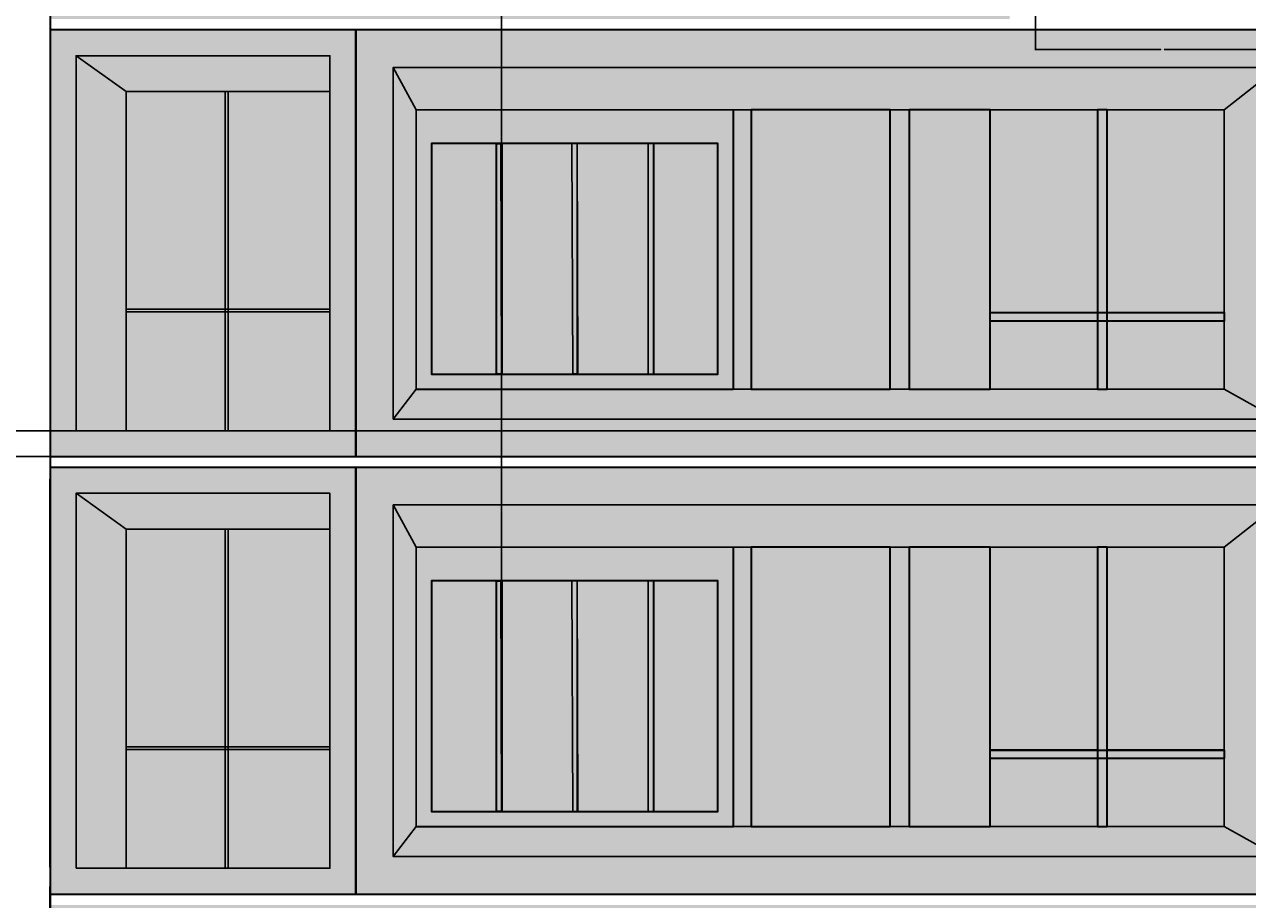
# Model space of a CAD drawing. Units: feet. Extents: x 1141 to 2858, y 751 to 1654.
# Tile 5 of 13: x 1718 to 2096, y 1195 to 1466. Entities that reach past the tile are written whole.
import ezdxf

# ---------------------------------------------------------------- set-up
doc = ezdxf.new("R2010")
doc.units = ezdxf.units.FT
for name, color, linetype, lineweight in [('A-ANNO-DIMS', 2, 'Continuous', 18), ('A-ELEV', 7, 'Continuous', 35), ('A-ELEV-PATT', 8, 'Continuous', 13), ('A-GLAZ', 4, 'Continuous', 25)]:
    doc.layers.add(name, color=color, linetype=linetype, lineweight=lineweight)
doc.styles.get("Standard").update_dxf_attribs({"font": 'arial.ttf'})
doc.dimstyles.get("Standard").update_dxf_attribs({"dimtxt": 0.18, "dimasz": 0.18, "dimexe": 0.18, "dimexo": 0.0625, "dimgap": 0.09, "dimtad": 0, "dimtih": 1, "dimtoh": 1, "dimdec": 1, "dimzin": 0, "dimdsep": 46, "dimlunit": 3, "dimtxsty": 'Standard', "dimcen": 0.09, "dimadec": 0, "dimazin": 0, "dimtfac": 1, "dimtdec": 1, "dimtofl": 0, "dimtmove": 0, "dimatfit": 3, "dimfxl": 1, "dimtolj": 1, "dimtzin": 0, "dimarcsym": 0})

# ---------------------------------------------------------------- blocks, each defined once
blk = doc.blocks.new('WIN-SIDE-A')
blk.add_line((63.09, 104.94), (78.57, 116.03))
blk.add_line((63.09, 104.94), (78.57, 116.03))
for points in [[(78.57, 0), (0, 0), (0, 116.03), (78.57, 116.03)], [(78.57, 0), (0, 0), (0, 116.03), (78.57, 116.03)], [(31.54, 104.94), (32.46, 104.94), (32.46, 0), (31.54, 0)], [(0, 37.61), (63.09, 37.61), (63.09, 36.79), (0, 36.79)]]:
    blk.add_lwpolyline(points, close=True)
for points in [[(63.09, 0), (63.09, 104.94), (0, 104.94)], [(63.09, 0), (63.09, 104.94), (0, 104.94)], [(31.54, 37.61), (31.54, 104.94), (32.46, 104.94), (32.46, 37.61)], [(31.54, 36.79), (0, 36.79), (0, 37.61), (31.54, 37.61)], [(32.46, 36.79), (32.46, 0), (31.54, 0), (31.54, 36.79)], [(32.46, 37.61), (63.09, 37.61), (63.09, 36.79), (32.46, 36.79)]]:
    blk.add_lwpolyline(points)
blk = doc.blocks.new('BALCONY-GLAZ-A')
for p, q in [((0, 108.84), (16.63, 95.74)), ((0, 108.84), (16.63, 95.74)), ((266.62, 95.74), (273.67, 108.84)), ((266.62, 95.74), (273.67, 108.84)), ((16.63, 95.74), (16.63, 9.29)), ((16.63, 95.74), (266.62, 95.74)), ((16.63, 95.74), (16.63, 9.29)), ((16.63, 95.74), (266.62, 95.74)), ((266.62, 95.74), (266.62, 9.19)), ((266.62, 95.74), (266.62, 9.19)), ((16.63, 9.29), (0, 0)), ((16.63, 9.29), (0, 0)), ((16.63, 9.29), (266.62, 9.29)), ((16.63, 9.29), (266.62, 9.29)), ((266.62, 9.29), (273.67, 0)), ((266.62, 9.29), (273.67, 0))]:
    blk.add_line(p, q)
for points in [[(0, 108.84), (273.67, 108.84), (273.67, 0), (0, 0)], [(0, 108.84), (273.67, 108.84), (273.67, 0), (0, 0)], [(266.62, 9.19), (168.47, 9.19), (168.47, 95.74), (266.62, 95.74)], [(266.62, 9.19), (168.47, 9.19), (168.47, 95.74), (266.62, 95.74)]]:
    blk.add_lwpolyline(points, close=True)
blk = doc.blocks.new('WIN-SLIDING')
for points in [[(36.16, 23.71), (36.16, 86.44), (39.2, 86.44), (39.2, 23.71)], [(36.16, 23.71), (0, 23.71), (0, 21.05), (36.16, 21.05)], [(39.2, 21.05), (72.32, 21.05), (72.32, 23.71), (39.2, 23.71)], [(39.2, 21.05), (39.2, 0), (36.16, 0), (36.16, 21.05)]]:
    blk.add_lwpolyline(points)
blk = doc.blocks.new('GLAZ-PANEL-A')
blk.add_lwpolyline([(1.57, 71.37), (0, 71.37), (0, 0), (1.57, 0)], close=True)
for points in [[(1.57, 71.37), (23.57, 71.37)], [(1.57, 0), (1.57, 71.37)], [(23.57, 71.37), (23.57, 0)], [(23.57, 0), (1.57, 0)]]:
    blk.add_lwpolyline(points)
blk = doc.blocks.new('*D15')
at = {"layer": 'A-ANNO-DIMS', "color": 0, "lineweight": -2, "transparency": 16777216}
for p, q in [((2030.85, 1475.38), (2030.85, 1457.85)), ((2109.42, 1475.38), (2109.42, 1457.85)), ((2031.03, 1458.03), (2069.61, 1458.03)), ((2109.24, 1458.03), (2070.66, 1458.03))]:
    blk.add_line(p, q, dxfattribs=at)
at = {"layer": 'A-ANNO-DIMS', "color": 0, "transparency": 16777216}
for points in [[(2031.03, 1458.06), (2031.03, 1458), (2030.85, 1458.03)], [(2109.24, 1458.06), (2109.24, 1458), (2109.42, 1458.03)]]:
    blk.add_solid(points, dxfattribs=at)
at = {"layer": 'Defpoints', "color": 0, "transparency": 16777216}
for p in [(2030.85, 1475.44), (2109.42, 1475.44), (2109.42, 1458.03)]:
    blk.add_point(p, dxfattribs=at)
at = {"layer": 'A-ANNO-DIMS', "color": 0, "transparency": 16777216, "insert": (2070.14, 1458.03), "char_height": 0.18, "attachment_point": 5}
blk.add_mtext('\\A1;79 TYP.', dxfattribs=at)
blk = doc.blocks.new('*D24')
at = {"layer": 'A-ANNO-DIMS', "color": 0, "lineweight": -2, "transparency": 16777216}
for p, q in [((1725.97, 1599.45), (1668.14, 1599.45)), ((1668.32, 1599.27), (1668.32, 1202.86)), ((1668.32, 806.08), (1668.32, 1202.49)), ((1725.97, 805.9), (1668.14, 805.9))]:
    blk.add_line(p, q, dxfattribs=at)
at = {"layer": 'A-ANNO-DIMS', "color": 0, "transparency": 16777216}
for points in [[(1668.29, 1599.27), (1668.35, 1599.27), (1668.32, 1599.45)], [(1668.29, 806.08), (1668.35, 806.08), (1668.32, 805.9)]]:
    blk.add_solid(points, dxfattribs=at)
at = {"layer": 'Defpoints', "color": 0, "transparency": 16777216}
for p in [(1668.32, 1599.45), (1726.03, 1599.45), (1726.03, 805.9)]:
    blk.add_point(p, dxfattribs=at)
at = {"layer": 'A-ANNO-DIMS', "color": 0, "transparency": 16777216, "insert": (1668.32, 1202.68), "char_height": 0.18, "attachment_point": 5}
blk.add_mtext('\\A1;793.6', dxfattribs=at)
blk = doc.blocks.new('*D39')
at = {"layer": 'A-ANNO-DIMS', "color": 0, "lineweight": -2, "transparency": 16777216}
for p, q in [((2319.24, 1599.45), (1668.14, 1599.45)), ((1668.32, 1599.27), (1668.32, 1202.86)), ((1668.32, 806.08), (1668.32, 1202.49)), ((2319.24, 805.9), (1668.14, 805.9))]:
    blk.add_line(p, q, dxfattribs=at)
at = {"layer": 'A-ANNO-DIMS', "color": 0, "transparency": 16777216}
for points in [[(1668.29, 1599.27), (1668.35, 1599.27), (1668.32, 1599.45)], [(1668.29, 806.08), (1668.35, 806.08), (1668.32, 805.9)]]:
    blk.add_solid(points, dxfattribs=at)
at = {"layer": 'Defpoints', "color": 0, "transparency": 16777216}
for p in [(1668.32, 1599.45), (2319.3, 1599.45), (2319.3, 805.9)]:
    blk.add_point(p, dxfattribs=at)
at = {"layer": 'A-ANNO-DIMS', "color": 0, "transparency": 16777216, "insert": (1668.32, 1202.68), "char_height": 0.18, "attachment_point": 5}
blk.add_mtext('\\A1;793.6', dxfattribs=at)
blk = doc.blocks.new('*D54')
at = {"layer": 'A-ANNO-DIMS', "color": 0, "lineweight": -2, "transparency": 16777216}
for p, q in [((2327.22, 1340.05), (1668.14, 1340.05)), ((1668.32, 1339.87), (1668.32, 1336.24)), ((1668.32, 1332.24), (1668.32, 1335.88)), ((2319.24, 1332.06), (1668.14, 1332.06))]:
    blk.add_line(p, q, dxfattribs=at)
at = {"layer": 'A-ANNO-DIMS', "color": 0, "transparency": 16777216}
for points in [[(1668.29, 1339.87), (1668.35, 1339.87), (1668.32, 1340.05)], [(1668.29, 1332.24), (1668.35, 1332.24), (1668.32, 1332.06)]]:
    blk.add_solid(points, dxfattribs=at)
at = {"layer": 'Defpoints', "color": 0, "transparency": 16777216}
for p in [(1668.32, 1340.05), (2327.29, 1340.05), (2319.3, 1332.06)]:
    blk.add_point(p, dxfattribs=at)
at = {"layer": 'A-ANNO-DIMS', "color": 0, "transparency": 16777216, "insert": (1668.32, 1336.06), "char_height": 0.18, "attachment_point": 5}
blk.add_mtext('\\A1;7.986', dxfattribs=at)
blk = doc.blocks.new('*D91')
at = {"layer": 'A-ANNO-DIMS', "color": 0, "lineweight": -2, "transparency": 16777216}
for p, q in [((1726.03, 1196.74), (1726.03, 1654.28)), ((1726.21, 1654.1), (1795.4, 1654.1)), ((1865.51, 1654.1), (1796.32, 1654.1)), ((1865.69, 1222.22), (1865.69, 1654.28))]:
    blk.add_line(p, q, dxfattribs=at)
at = {"layer": 'A-ANNO-DIMS', "color": 0, "transparency": 16777216}
for points in [[(1726.21, 1654.13), (1726.21, 1654.07), (1726.03, 1654.1)], [(1865.51, 1654.13), (1865.51, 1654.07), (1865.69, 1654.1)]]:
    blk.add_solid(points, dxfattribs=at)
at = {"layer": 'Defpoints', "color": 0, "transparency": 16777216}
for p in [(1865.69, 1654.1), (1865.69, 1222.16), (1726.03, 1196.68)]:
    blk.add_point(p, dxfattribs=at)
at = {"layer": 'A-ANNO-DIMS', "color": 0, "transparency": 16777216, "insert": (1795.86, 1654.1), "char_height": 0.18, "attachment_point": 5}
blk.add_mtext('\\A1;139.65', dxfattribs=at)

msp = doc.modelspace()

# ---------------------------------------------------------------- hatches: boundary and pattern name
at = {"layer": 'A-ELEV-PATT'}
h = msp.add_hatch(color=256, dxfattribs=at)
h.dxf.hatch_style = 1
h.paths.add_polyline_path([(2206.032, 1599.4527), (2192.689, 1599.4527), (2192.689, 919.339), (2206.032, 919.339)])
h.paths.add_polyline_path([(2190.2416, 1599.4527), (2175.463, 1599.4527), (2175.463, 919.339), (2190.2416, 919.339)])
h.paths.add_polyline_path([(2173.0156, 1599.4527), (2117.407, 1599.4527), (2117.407, 919.339), (2173.0156, 919.339)])
h.paths.add_polyline_path([(2022.8666, 1057.9008), (1726.032, 1057.9008), (1726.032, 925.9008), (2022.8666, 925.9008)])
h.paths.add_polyline_path([(1737.6123, 937.4811), (1737.6123, 1046.3205), (2011.2863, 1046.3205), (2011.2863, 937.4811)], flags=16)
h.paths.add_polyline_path([(1754.2423, 946.7736), (1754.2423, 1033.2183), (2004.2323, 1033.2183), (2004.2323, 946.7736), (2004.3069, 946.6754), (1906.0824, 946.6754)], flags=0)
h.paths.add_polyline_path([(1900.5421, 946.7736), (1857.5566, 946.7736), (1857.5566, 1033.2183), (1900.5421, 1033.2183)], flags=0)
h.paths.add_polyline_path([(1910.8368, 951.4297), (1910.8368, 1022.7957), (1999.478, 1022.7957), (1999.478, 951.4297)], flags=0)
h.paths.add_polyline_path([(1930.8039, 951.4297), (1930.8039, 1022.7957), (1932.373, 1022.7957), (1932.373, 951.4297)], flags=0)
h.paths.add_polyline_path([(1851.6414, 946.7736), (1826.5664, 946.7736), (1826.5664, 967.8234), (1793.4402, 967.8234), (1793.4402, 946.7736), (1790.4043, 946.7736), (1790.4043, 967.8234), (1754.2423, 967.8234), (1754.2423, 970.4796), (1790.4043, 970.4796), (1790.4043, 1033.2183), (1793.4402, 1033.2183), (1793.4402, 970.4796), (1826.5664, 970.4796), (1826.5664, 1033.2183), (1851.6414, 1033.2183)], flags=0)
h.paths.add_polyline_path([(1954.3728, 951.4297), (1954.3728, 1022.7957), (1955.9419, 1022.7957), (1955.9419, 951.4297)], flags=0)
h.paths.add_polyline_path([(1977.7327, 951.4297), (1977.7327, 1022.7957), (1979.3018, 1022.7957), (1979.3018, 951.4297)], flags=0)
h.paths.add_polyline_path([(2022.8666, 1193.2888), (1726.032, 1193.2888), (1726.032, 1061.2888), (2022.8666, 1061.2888)])
h.paths.add_polyline_path([(1737.6123, 1072.869), (1737.6123, 1181.7085), (2011.2863, 1181.7085), (2011.2863, 1072.869)], flags=16)
h.paths.add_polyline_path([(1754.2423, 1082.1616), (1754.2423, 1168.6063), (2004.2323, 1168.6063), (2004.2323, 1082.1616), (2004.3069, 1082.0634), (1906.0824, 1082.0634)], flags=0)
h.paths.add_polyline_path([(1900.5421, 1082.1616), (1857.5566, 1082.1616), (1857.5566, 1168.6063), (1900.5421, 1168.6063)], flags=0)
h.paths.add_polyline_path([(1910.8368, 1086.8177), (1910.8368, 1158.1837), (1999.478, 1158.1837), (1999.478, 1086.8177)], flags=0)
h.paths.add_polyline_path([(1930.8039, 1086.8177), (1930.8039, 1158.1837), (1932.373, 1158.1837), (1932.373, 1086.8177)], flags=0)
h.paths.add_polyline_path([(1851.6414, 1082.1616), (1826.5664, 1082.1616), (1826.5664, 1103.2114), (1793.4402, 1103.2114), (1793.4402, 1082.1616), (1790.4043, 1082.1616), (1790.4043, 1103.2114), (1754.2423, 1103.2114), (1754.2423, 1105.8676), (1790.4043, 1105.8676), (1790.4043, 1168.6063), (1793.4402, 1168.6063), (1793.4402, 1105.8676), (1826.5664, 1105.8676), (1826.5664, 1168.6063), (1851.6414, 1168.6063)], flags=0)
h.paths.add_polyline_path([(1954.3728, 1086.8177), (1954.3728, 1158.1837), (1955.9419, 1158.1837), (1955.9419, 1086.8177)], flags=0)
h.paths.add_polyline_path([(1977.7327, 1086.8177), (1977.7327, 1158.1837), (1979.3018, 1158.1837), (1979.3018, 1086.8177)], flags=0)
h.paths.add_polyline_path([(2022.8666, 1599.4527), (1726.032, 1599.4527), (1726.032, 1467.4527), (2022.8666, 1467.4527)])
h.paths.add_polyline_path([(2011.2863, 1479.033), (1737.6123, 1479.033), (1737.6123, 1587.8725), (2011.2863, 1587.8725)], flags=16)
h.paths.add_polyline_path([(2004.2323, 1488.3255), (1754.2423, 1488.3255), (1754.2423, 1574.7702), (2004.2323, 1574.7702)], flags=0)
h.paths.add_polyline_path([(1829.1345, 1544.6458), (1914.1177, 1544.6458), (1914.1177, 1539.5463), (1830.9097, 1539.5463), (1831.6817, 1537.3286), (1914.1177, 1537.3286), (1914.1177, 1532.2291), (1833.4569, 1532.2291), (1834.229, 1530.0113), (1914.1177, 1530.0113), (1914.1177, 1524.9118), (1836.0042, 1524.9118), (1836.7762, 1522.694), (1914.1177, 1522.694), (1914.1177, 1517.5946), (1838.5514, 1517.5946), (1839.3235, 1515.3768), (1914.1177, 1515.3768), (1914.1177, 1510.2773), (1841.0987, 1510.2773), (1841.8707, 1508.0595), (1914.1177, 1508.0595), (1914.1177, 1502.9601), (1843.6459, 1502.9601), (1844.4179, 1500.7423), (1914.1177, 1500.7423), (1914.1177, 1495.6428), (1846.1931, 1495.6428), (1846.9652, 1493.425), (1914.1177, 1493.425), (1914.1177, 1488.3255), (1848.6593, 1488.3255), (1848.6593, 1488.5583)], flags=0)
h.paths.add_polyline_path([(2117.407, 1464.0647), (1820.5724, 1464.0647), (1820.5724, 1332.0647), (2117.407, 1332.0647)])
h.paths.add_polyline_path([(2105.8267, 1452.4845), (2105.8267, 1343.645), (1832.1527, 1343.645), (1832.1527, 1452.4845)], flags=16)
h.paths.add_polyline_path([(2089.1967, 1439.3822), (2089.1967, 1352.9376), (1937.3566, 1352.9376), (1937.3566, 1352.8393), (1839.1321, 1352.8393), (1839.2067, 1352.9376), (1839.2067, 1439.3822), (1937.3566, 1439.3822)], flags=0)
h.paths.add_polyline_path([(2016.8727, 1439.3822), (2016.8727, 1376.6436), (2049.9988, 1376.6436), (2049.9988, 1439.3822), (2053.0347, 1439.3822), (2053.0347, 1376.6436), (2089.1967, 1376.6436), (2089.1967, 1373.9873), (2053.0347, 1373.9873), (2053.0347, 1352.9376), (2049.9988, 1352.9376), (2049.9988, 1373.9873), (2016.8727, 1373.9873), (2016.8727, 1352.9376), (1991.7976, 1352.9376), (1991.7976, 1439.3822)], flags=0)
h.paths.add_polyline_path([(1985.8824, 1439.3822), (1985.8824, 1352.9376), (1942.8969, 1352.9376), (1942.8969, 1439.3822)], flags=0)
h.paths.add_polyline_path([(1932.6022, 1428.9596), (1932.6022, 1357.5937), (1843.961, 1357.5937), (1843.961, 1428.9596)], flags=0)
h.paths.add_polyline_path([(1912.6351, 1428.9596), (1912.6351, 1357.5937), (1911.066, 1357.5937), (1911.066, 1428.9596)], flags=0)
h.paths.add_polyline_path([(1889.0662, 1428.9596), (1889.0662, 1357.5937), (1887.4971, 1357.5937), (1887.4971, 1428.9596)], flags=0)
h.paths.add_polyline_path([(1865.7063, 1428.9596), (1865.7063, 1357.5937), (1864.1372, 1357.5937), (1864.1372, 1428.9596)], flags=0)
h.paths.add_polyline_path([(2117.407, 1328.6768), (1820.5724, 1328.6768), (1820.5724, 1196.6768), (2117.407, 1196.6768)])
h.paths.add_polyline_path([(2105.8267, 1317.0965), (2105.8267, 1208.257), (1832.1527, 1208.257), (1832.1527, 1317.0965)], flags=16)
h.paths.add_polyline_path([(2089.1967, 1303.9943), (2089.1967, 1217.5496), (1937.3566, 1217.5496), (1937.3566, 1217.4513), (1839.1321, 1217.4513), (1839.2067, 1217.5496), (1839.2067, 1303.9943), (1937.3566, 1303.9943)], flags=0)
h.paths.add_polyline_path([(2016.8727, 1303.9943), (2016.8727, 1241.2556), (2049.9988, 1241.2556), (2049.9988, 1303.9943), (2053.0347, 1303.9943), (2053.0347, 1241.2556), (2089.1967, 1241.2556), (2089.1967, 1238.5993), (2053.0347, 1238.5993), (2053.0347, 1217.5496), (2049.9988, 1217.5496), (2049.9988, 1238.5993), (2016.8727, 1238.5993), (2016.8727, 1217.5496), (1991.7976, 1217.5496), (1991.7976, 1303.9943)], flags=0)
h.paths.add_polyline_path([(1985.8824, 1303.9943), (1985.8824, 1217.5496), (1942.8969, 1217.5496), (1942.8969, 1303.9943)], flags=0)
h.paths.add_polyline_path([(1932.6022, 1293.5716), (1932.6022, 1222.2057), (1843.961, 1222.2057), (1843.961, 1293.5716)], flags=0)
h.paths.add_polyline_path([(1912.6351, 1293.5716), (1912.6351, 1222.2057), (1911.066, 1222.2057), (1911.066, 1293.5716)], flags=0)
h.paths.add_polyline_path([(1889.0662, 1293.5716), (1889.0662, 1222.2057), (1887.4971, 1222.2057), (1887.4971, 1293.5716)], flags=0)
h.paths.add_polyline_path([(1865.7063, 1293.5716), (1865.7063, 1222.2057), (1864.1372, 1222.2057), (1864.1372, 1293.5716)], flags=0)
h.paths.add_polyline_path([(2206.032, 917.3598), (2027.2589, 917.3598), (2027.2589, 805.9008), (2206.032, 805.9008)])
h.paths.add_polyline_path([(1852.1771, 917.3598), (1726.032, 917.3598), (1726.032, 805.9008), (1852.1771, 805.9008)])
h.paths.add_polyline_path([(2063.3101, 1580.3829), (2093.938, 1580.3829), (2093.938, 1513.0494), (2063.3101, 1513.0494)])
h.paths.add_polyline_path([(2063.3101, 1580.3829), (2093.938, 1580.3829), (2093.938, 1513.0494), (2063.3101, 1513.0494)])
h = msp.add_hatch(color=256, dxfattribs=at)
h.dxf.hatch_style = 1
h.paths.add_polyline_path([(2011.2863, 1587.8725), (1737.6123, 1587.8725), (1754.2423, 1574.7702), (2004.2323, 1574.7702)])
h.paths.add_polyline_path([(1754.2423, 1574.7702), (1737.6123, 1587.8725), (1737.6123, 1479.033), (1754.2423, 1488.3255)])
h.paths.add_polyline_path([(2011.2863, 1587.8725), (2004.2323, 1574.7702), (2004.2323, 1488.3255), (2011.2863, 1479.033)])
h.paths.add_polyline_path([(2004.2323, 1488.3255), (1754.2423, 1488.3255), (1737.6123, 1479.033), (2011.2863, 1479.033)])
h.paths.add_polyline_path([(2105.8267, 1452.4845), (1832.1527, 1452.4845), (1839.2067, 1439.3822), (1937.3566, 1439.3822), (2089.1967, 1439.3822)])
h.paths.add_polyline_path([(1839.2067, 1439.3822), (1832.1527, 1452.4845), (1832.1527, 1343.645), (1839.2067, 1352.9376)])
h.paths.add_polyline_path([(2105.8267, 1452.4845), (2089.1967, 1439.3822), (2089.1967, 1352.9376), (2105.8267, 1343.645)])
h.paths.add_polyline_path([(2089.1967, 1352.9376), (1937.3566, 1352.9376), (1937.3566, 1352.8393), (1839.1321, 1352.8393), (1832.1527, 1343.645), (2105.8267, 1343.645)])
h.paths.add_polyline_path([(1942.8969, 1439.3822), (1937.3566, 1439.3822), (1937.3566, 1352.9376), (1942.8969, 1352.9376)])
h.paths.add_polyline_path([(1991.7976, 1439.3822), (1985.8824, 1439.3822), (1985.8824, 1352.9376), (1991.7976, 1352.9376)])
h.paths.add_polyline_path([(2109.4211, 1591.4669), (2030.8524, 1591.4669), (2030.8524, 1580.3829), (2093.938, 1580.3829)])
h.paths.add_polyline_path([(2109.4211, 1591.4669), (2093.938, 1580.3829), (2093.938, 1475.4386), (2109.4211, 1475.4386)])
h.paths.add_polyline_path([(1991.7976, 1303.9943), (1985.8824, 1303.9943), (1985.8824, 1217.5496), (1991.7976, 1217.5496)])
h.paths.add_polyline_path([(1942.8969, 1303.9943), (1937.3566, 1303.9943), (1937.3566, 1217.5496), (1942.8969, 1217.5496)])
h.paths.add_polyline_path([(2105.8267, 1317.0965), (1832.1527, 1317.0965), (1839.2067, 1303.9943), (1937.3566, 1303.9943), (2089.1967, 1303.9943)])
h.paths.add_polyline_path([(1839.2067, 1303.9943), (1832.1527, 1317.0965), (1832.1527, 1208.257), (1839.2067, 1217.5496)])
h.paths.add_polyline_path([(2089.1967, 1217.5496), (1937.3566, 1217.5496), (1937.3566, 1217.4513), (1839.1321, 1217.4513), (1832.1527, 1208.257), (2105.8267, 1208.257)])
h.paths.add_polyline_path([(2105.8267, 1317.0965), (2089.1967, 1303.9943), (2089.1967, 1217.5496), (2105.8267, 1208.257)])
h.paths.add_polyline_path([(1754.2423, 1168.6063), (1737.6123, 1181.7085), (1737.6123, 1072.869), (1754.2423, 1082.1616)])
h.paths.add_polyline_path([(2011.2863, 1181.7085), (1737.6123, 1181.7085), (1754.2423, 1168.6063), (2004.2323, 1168.6063)])
h.paths.add_polyline_path([(2011.2863, 1181.7085), (2004.2323, 1168.6063), (2004.2323, 1082.1616), (2011.2863, 1072.869)])
h.paths.add_polyline_path([(2004.3069, 1082.0634), (1906.0824, 1082.0634), (1754.2423, 1082.1616), (1737.6123, 1072.869), (2011.2863, 1072.869)])
h.paths.add_polyline_path([(1906.0824, 1168.6063), (1900.5421, 1168.6063), (1900.5421, 1082.1616), (1906.0824, 1082.1616)])
h.paths.add_polyline_path([(1857.5566, 1168.6063), (1851.6414, 1168.6063), (1851.6414, 1082.1616), (1857.5566, 1082.1616)])
h.paths.add_polyline_path([(1906.0824, 1033.2183), (1900.5421, 1033.2183), (1900.5421, 946.7736), (1906.0824, 946.7736)])
h.paths.add_polyline_path([(1857.5566, 1033.2183), (1851.6414, 1033.2183), (1851.6414, 946.7736), (1857.5566, 946.7736)])
h.paths.add_polyline_path([(1754.2423, 1033.2183), (1737.6123, 1046.3205), (1737.6123, 937.4811), (1754.2423, 946.7736)])
h.paths.add_polyline_path([(2011.2863, 1046.3205), (1737.6123, 1046.3205), (1754.2423, 1033.2183), (2004.2323, 1033.2183)])
h.paths.add_polyline_path([(2011.2863, 1046.3205), (2004.2323, 1033.2183), (2004.2323, 946.7736), (2011.2863, 937.4811)])
h.paths.add_polyline_path([(2004.3069, 946.6754), (1906.0824, 946.6754), (1754.2423, 946.7736), (1737.6123, 937.4811), (2011.2863, 937.4811)])
h.paths.add_polyline_path([(2175.463, 1599.4527), (2173.0156, 1599.4527), (2173.0156, 919.339), (2175.463, 919.339)])
h = msp.add_hatch(color=256, dxfattribs=at)
h.dxf.hatch_style = 1
h.paths.add_polyline_path([(2062.3952, 1580.3829), (2030.8524, 1580.3829), (2030.8524, 1513.0494), (2062.3952, 1513.0494)])
h.paths.add_polyline_path([(2093.938, 1580.3829), (2063.3101, 1580.3829), (2063.3101, 1513.0494), (2093.938, 1513.0494)])
h.paths.add_polyline_path([(2093.938, 1512.23), (2063.3101, 1512.23), (2063.3101, 1475.4386), (2093.938, 1475.4386)])
h.paths.add_polyline_path([(2062.3952, 1512.23), (2030.8524, 1512.23), (2030.8524, 1475.4386), (2062.3952, 1475.4386)])
h.paths.add_polyline_path([(1780.1289, 1444.9949), (1749.501, 1444.9949), (1749.501, 1377.6615), (1780.1289, 1377.6615)])
h.paths.add_polyline_path([(1812.5866, 1444.9949), (1781.0438, 1444.9949), (1781.0438, 1377.6615), (1812.5866, 1377.6615)])
h.paths.add_polyline_path([(1812.5866, 1376.842), (1781.0438, 1376.842), (1781.0438, 1340.0506), (1812.5866, 1340.0506)])
h.paths.add_polyline_path([(1780.1289, 1376.842), (1749.501, 1376.842), (1749.501, 1340.0506), (1780.1289, 1340.0506)])
h.paths.add_polyline_path([(2105.8267, 1452.4845), (1832.1527, 1452.4845), (1832.1527, 1343.645), (1839.2067, 1352.9376), (1839.2067, 1439.3822), (1937.3566, 1439.3822), (1937.3566, 1352.9376), (1942.8969, 1352.9376), (1942.8969, 1439.3822), (1985.8824, 1439.3822), (1985.8824, 1352.9376), (1991.7976, 1352.9376), (1991.7976, 1439.3822), (2016.8727, 1439.3822), (2016.8727, 1376.6436), (2049.9988, 1376.6436), (2049.9988, 1439.3822), (2053.0347, 1439.3822), (2053.0347, 1376.6436), (2089.1967, 1376.6436), (2089.1967, 1373.9873), (2053.0347, 1373.9873), (2053.0347, 1352.9376), (2049.9988, 1352.9376), (1937.3566, 1352.9376), (1937.3566, 1352.8393), (1839.1321, 1352.8393), (1832.1527, 1343.645), (2105.8267, 1343.645)])
h.paths.add_polyline_path([(2049.9988, 1373.9873), (2016.8727, 1373.9873), (2016.8727, 1352.9376), (2049.9988, 1352.9376)], flags=17)
h.paths.add_polyline_path([(1780.1289, 1309.6069), (1749.501, 1309.6069), (1749.501, 1242.2735), (1780.1289, 1242.2735)])
h.paths.add_polyline_path([(1812.5866, 1309.6069), (1781.0438, 1309.6069), (1781.0438, 1242.2735), (1812.5866, 1242.2735)])
h.paths.add_polyline_path([(1812.5866, 1241.454), (1781.0438, 1241.454), (1781.0438, 1204.6626), (1812.5866, 1204.6626)])
h.paths.add_polyline_path([(1780.1289, 1241.454), (1749.501, 1241.454), (1749.501, 1204.6626), (1780.1289, 1204.6626)])
h.paths.add_polyline_path([(2049.9988, 1303.9943), (2016.8727, 1303.9943), (2016.8727, 1241.2556), (2049.9988, 1241.2556)])
h.paths.add_polyline_path([(2089.1967, 1303.9943), (2053.0347, 1303.9943), (2053.0347, 1241.2556), (2089.1967, 1241.2556)])
h.paths.add_polyline_path([(2089.1967, 1238.5993), (2053.0347, 1238.5993), (2053.0347, 1217.5496), (2089.1967, 1217.5496)])
h.paths.add_polyline_path([(2049.9988, 1238.5993), (2016.8727, 1238.5993), (2016.8727, 1217.5496), (2049.9988, 1217.5496)])
h.paths.add_polyline_path([(2062.3952, 1174.219), (2030.8524, 1174.219), (2030.8524, 1106.8855), (2062.3952, 1106.8855)])
h.paths.add_polyline_path([(2093.938, 1174.219), (2063.3101, 1174.219), (2063.3101, 1106.8855), (2093.938, 1106.8855)])
h.paths.add_polyline_path([(2093.938, 1106.066), (2063.3101, 1106.066), (2063.3101, 1069.2747), (2093.938, 1069.2747)])
h.paths.add_polyline_path([(2062.3952, 1106.066), (2030.8524, 1106.066), (2030.8524, 1069.2747), (2062.3952, 1069.2747)])
h.paths.add_polyline_path([(1906.0824, 1168.6063), (2004.2323, 1168.6063), (2011.2863, 1181.7085), (1737.6123, 1181.7085), (1737.6123, 1072.869), (2011.2863, 1072.869), (2004.3069, 1082.0634), (1906.0824, 1082.0634)])
h.paths.add_polyline_path([(1790.4043, 1168.6063), (1793.4402, 1168.6063), (1793.4402, 1105.8676), (1826.5664, 1105.8676), (1826.5664, 1168.6063), (1851.6414, 1168.6063), (1851.6414, 1082.1616), (1826.5664, 1082.1616), (1826.5664, 1103.2114), (1793.4402, 1103.2114), (1793.4402, 1082.1616), (1790.4043, 1082.1616), (1790.4043, 1103.2114), (1754.2423, 1103.2114), (1754.2423, 1105.8676), (1790.4043, 1105.8676)], flags=16)
h.paths.add_polyline_path([(1857.5566, 1168.6063), (1900.5421, 1168.6063), (1900.5421, 1082.1616), (1857.5566, 1082.1616)], flags=16)
h = msp.add_hatch(color=256, dxfattribs=at)
h.dxf.hatch_style = 1
h.paths.add_polyline_path([(1812.5866, 1456.0789), (1734.0179, 1456.0789), (1749.501, 1444.9949), (1812.5866, 1444.9949)], flags=0)
h.paths.add_polyline_path([(1820.5724, 1464.0647), (1726.032, 1464.0647), (1726.032, 1332.0647), (1820.5724, 1332.0647)])
h.paths.add_polyline_path([(1734.0179, 1456.0789), (1812.5866, 1456.0789), (1812.5866, 1340.0506), (1734.0179, 1340.0506)], flags=16)
h.paths.add_polyline_path([(1749.501, 1444.9949), (1781.0438, 1444.9949), (1781.0438, 1377.6615), (1812.5866, 1377.6615), (1812.5866, 1376.842), (1781.0438, 1376.842), (1781.0438, 1340.0506), (1780.1289, 1340.0506), (1780.1289, 1376.842), (1749.501, 1376.842), (1749.501, 1377.6615)], flags=0)
h.paths.add_polyline_path([(1749.501, 1444.9949), (1734.0179, 1456.0789), (1734.0179, 1340.0506), (1749.501, 1340.0506)], flags=0)
h.paths.add_polyline_path([(1820.5724, 1328.6768), (1726.032, 1328.6768), (1726.032, 1196.6768), (1820.5724, 1196.6768)])
h.paths.add_polyline_path([(1734.0179, 1320.6909), (1812.5866, 1320.6909), (1812.5866, 1204.6626), (1734.0179, 1204.6626)], flags=16)
h.paths.add_polyline_path([(1749.501, 1309.6069), (1781.0438, 1309.6069), (1781.0438, 1242.2735), (1812.5866, 1242.2735), (1812.5866, 1241.454), (1781.0438, 1241.454), (1781.0438, 1204.6626), (1780.1289, 1204.6626), (1780.1289, 1241.454), (1749.501, 1241.454), (1749.501, 1242.2735)], flags=0)
h.paths.add_polyline_path([(1749.501, 1309.6069), (1734.0179, 1320.6909), (1734.0179, 1204.6626), (1749.501, 1204.6626)], flags=0)
h.paths.add_polyline_path([(2117.407, 1193.2888), (2022.8666, 1193.2888), (2022.8666, 1061.2888), (2117.407, 1061.2888)])
h.paths.add_polyline_path([(2109.4211, 1185.3029), (2109.4211, 1069.2747), (2030.8524, 1069.2747), (2030.8524, 1185.3029)], flags=16)
h.paths.add_polyline_path([(2093.938, 1174.219), (2093.938, 1106.066), (2063.3101, 1106.066), (2063.3101, 1069.2747), (2062.3952, 1069.2747), (2062.3952, 1106.066), (2030.8524, 1106.066), (2030.8524, 1106.8855), (2062.3952, 1106.8855), (2062.3952, 1174.219), (2063.3101, 1174.219)], flags=0)
h.paths.add_polyline_path([(2702.6903, 1049.9149), (2624.1217, 1049.9149), (2624.1217, 1038.831), (2687.2072, 1038.831), (2687.2072, 933.8867), (2702.6903, 933.8867)], flags=0)
h.paths.add_polyline_path([(2109.4211, 1049.9149), (2093.938, 1038.831), (2093.938, 933.8867), (2109.4211, 933.8867)])
h.paths.add_polyline_path([(2109.4211, 1049.9149), (2030.8524, 1049.9149), (2030.8524, 1038.831), (2093.938, 1038.831)])
h = msp.add_hatch(color=256, dxfattribs=at)
h.dxf.hatch_style = 1
h.paths.add_polyline_path([(1219.3173, 1456.0789), (1140.7487, 1456.0789), (1156.2318, 1444.9949), (1219.3173, 1444.9949)], flags=0)
h.paths.add_polyline_path([(1156.2318, 1444.9949), (1140.7487, 1456.0789), (1140.7487, 1340.0506), (1156.2318, 1340.0506)], flags=0)
h.paths.add_polyline_path([(1156.2318, 1309.6069), (1187.7746, 1309.6069), (1187.7746, 1242.2735), (1219.3173, 1242.2735), (1219.3173, 1241.454), (1187.7746, 1241.454), (1187.7746, 1204.6626), (1186.8597, 1204.6626), (1186.8597, 1241.454), (1156.2318, 1241.454), (1156.2318, 1242.2735)], flags=0)
h.paths.add_polyline_path([(2109.4211, 1049.9149), (2030.8524, 1049.9149), (2030.8524, 1038.831), (2093.938, 1038.831), (2093.938, 933.8867), (2109.4211, 933.8867)], flags=0)
h.paths.add_polyline_path([(2109.4211, 1185.3029), (2030.8524, 1185.3029), (2030.8524, 1174.219), (2093.938, 1174.219), (2093.938, 1069.2747), (2109.4211, 1069.2747)])
h.paths.add_polyline_path([(1812.5866, 1320.6909), (1734.0179, 1320.6909), (1749.501, 1309.6069), (1812.5866, 1309.6069)])
h.paths.add_polyline_path([(1749.501, 1309.6069), (1734.0179, 1320.6909), (1734.0179, 1204.6626), (1749.501, 1204.6626)])
h.paths.add_polyline_path([(1812.5866, 1456.0789), (1734.0179, 1456.0789), (1749.501, 1444.9949), (1812.5866, 1444.9949)])
h.paths.add_polyline_path([(2117.407, 1057.9008), (2022.8666, 1057.9008), (2022.8666, 925.9008), (2117.407, 925.9008)])
h.paths.add_polyline_path([(2030.8524, 933.8867), (2030.8524, 1049.9149), (2109.4211, 1049.9149), (2109.4211, 933.8867)], flags=16)
h.paths.add_polyline_path([(2062.3952, 933.8867), (2062.3952, 970.6781), (2030.8524, 970.6781), (2030.8524, 971.4975), (2062.3952, 971.4975), (2062.3952, 1038.831), (2063.3101, 1038.831), (2093.938, 1038.831), (2093.938, 970.6781), (2063.3101, 970.6781), (2063.3101, 933.8867)], flags=0)
h = msp.add_hatch(color=256, dxfattribs=at)
h.dxf.hatch_style = 1
h.paths.add_polyline_path([(1749.501, 1444.9949), (1734.0179, 1456.0789), (1734.0179, 1340.0506), (1749.501, 1340.0506)])
h = msp.add_hatch(color=256, dxfattribs=at)
h.dxf.hatch_style = 1
h.paths.add_polyline_path([(1812.5866, 1377.6615), (1781.0438, 1377.6615), (1781.0438, 1444.9949), (1780.1289, 1444.9949), (1780.1289, 1377.6615), (1749.501, 1377.6615), (1749.501, 1376.842), (1780.1289, 1376.842), (1780.1289, 1340.0506), (1781.0438, 1340.0506), (1781.0438, 1376.842), (1812.5866, 1376.842)])
h.paths.add_polyline_path([(2089.1967, 1241.2556), (2053.0347, 1241.2556), (2053.0347, 1303.9943), (2049.9988, 1303.9943), (2049.9988, 1241.2556), (2016.8727, 1241.2556), (2016.8727, 1238.5993), (2049.9988, 1238.5993), (2049.9988, 1217.5496), (2053.0347, 1217.5496), (2053.0347, 1238.5993), (2089.1967, 1238.5993)])
h.paths.add_polyline_path([(1937.3566, 1303.9943), (1839.2067, 1303.9943), (1839.2067, 1217.5496), (1937.3566, 1217.5496)])
h.paths.add_polyline_path([(1887.4971, 1293.5716), (1887.4971, 1222.2057), (1865.7063, 1222.2057), (1865.7063, 1293.5716)], flags=16)
h.paths.add_polyline_path([(1864.1372, 1293.5716), (1864.1372, 1222.2057), (1843.961, 1222.2057), (1843.961, 1293.5716)], flags=16)
h.paths.add_polyline_path([(1889.0662, 1293.5716), (1911.066, 1293.5716), (1911.066, 1222.2057), (1889.0662, 1222.2057)], flags=16)
h.paths.add_polyline_path([(1912.6351, 1293.5716), (1932.6022, 1293.5716), (1932.6022, 1222.2057), (1912.6351, 1222.2057)], flags=16)
h = msp.add_hatch(color=256, dxfattribs=at)
h.dxf.hatch_style = 1
h.paths.add_polyline_path([(2089.1967, 1376.6436), (2053.0347, 1376.6436), (2053.0347, 1439.3822), (2049.9988, 1439.3822), (2049.9988, 1376.6436), (2016.8727, 1376.6436), (2016.8727, 1373.9873), (2049.9988, 1373.9873), (2049.9988, 1352.9376), (2053.0347, 1352.9376), (2053.0347, 1373.9873), (2089.1967, 1373.9873)])
h.paths.add_polyline_path([(1937.3566, 1439.3822), (1839.2067, 1439.3822), (1839.2067, 1352.9376), (1937.3566, 1352.9376)])
h.paths.add_polyline_path([(1887.4971, 1428.9596), (1887.4971, 1357.5937), (1865.7063, 1357.5937), (1865.7063, 1428.9596)], flags=16)
h.paths.add_polyline_path([(1864.1372, 1428.9596), (1864.1372, 1357.5937), (1843.961, 1357.5937), (1843.961, 1428.9596)], flags=16)
h.paths.add_polyline_path([(1889.0662, 1428.9596), (1911.066, 1428.9596), (1911.066, 1357.5937), (1889.0662, 1357.5937)], flags=16)
h.paths.add_polyline_path([(1912.6351, 1428.9596), (1932.6022, 1428.9596), (1932.6022, 1357.5937), (1912.6351, 1357.5937)], flags=16)
h = msp.add_hatch(color=256, dxfattribs=at)
h.dxf.hatch_style = 1
h.paths.add_polyline_path([(1932.6022, 1428.9596), (1912.6351, 1428.9596), (1912.6351, 1357.5937), (1932.6022, 1357.5937)])
h.paths.add_polyline_path([(1864.1372, 1428.9596), (1843.961, 1428.9596), (1843.961, 1357.5937), (1864.1372, 1357.5937)])
h.paths.add_polyline_path([(1887.4971, 1428.9596), (1865.7063, 1428.9596), (1865.7063, 1357.5937), (1887.4971, 1357.5937)])
h.paths.add_polyline_path([(1911.066, 1428.9596), (1889.0662, 1428.9596), (1889.0662, 1357.5937), (1911.066, 1357.5937)])
h.paths.add_polyline_path([(2016.8727, 1439.3822), (1991.7976, 1439.3822), (1991.7976, 1352.9376), (2016.8727, 1352.9376)])
h = msp.add_hatch(color=256, dxfattribs=at)
h.dxf.hatch_style = 1
h.paths.add_polyline_path([(1985.8824, 1439.3822), (1942.8969, 1439.3822), (1942.8969, 1352.9376), (1985.8824, 1352.9376)])
h.paths.add_polyline_path([(1985.8824, 1303.9943), (1942.8969, 1303.9943), (1942.8969, 1217.5496), (1985.8824, 1217.5496)])
h.paths.add_polyline_path([(1900.5421, 1168.6063), (1857.5566, 1168.6063), (1857.5566, 1082.1616), (1900.5421, 1082.1616)])
h.paths.add_polyline_path([(1900.5421, 1033.2183), (1857.5566, 1033.2183), (1857.5566, 946.7736), (1900.5421, 946.7736)])
h = msp.add_hatch(color=256, dxfattribs=at)
h.dxf.hatch_style = 1
h.paths.add_polyline_path([(2089.1442, 1376.5731), (2052.9822, 1376.5731), (2052.9822, 1439.3118), (2049.9463, 1439.3118), (2049.9463, 1376.5731), (2016.8202, 1376.5731), (2016.8202, 1373.9168), (2049.9463, 1373.9168), (2049.9463, 1352.8671), (2052.9822, 1352.8671), (2052.9822, 1373.9168), (2089.1442, 1373.9168)])
h = msp.add_hatch(color=256, dxfattribs=at)
h.dxf.hatch_style = 1
h.paths.add_polyline_path([(1812.5821, 1242.2917), (1781.0393, 1242.2917), (1781.0393, 1309.6252), (1780.1245, 1309.6252), (1780.1245, 1242.2917), (1749.4966, 1242.2917), (1749.4966, 1241.4722), (1780.1245, 1241.4722), (1780.1245, 1204.6809), (1781.0393, 1204.6809), (1781.0393, 1241.4722), (1812.5821, 1241.4722)])
h = msp.add_hatch(color=256, dxfattribs=at)
h.dxf.hatch_style = 1
h.paths.add_polyline_path([(1812.5866, 1242.2735), (1781.0438, 1242.2735), (1781.0438, 1309.6069), (1780.1289, 1309.6069), (1780.1289, 1242.2735), (1749.501, 1242.2735), (1749.501, 1241.454), (1780.1289, 1241.454), (1780.1289, 1204.6626), (1781.0438, 1204.6626), (1781.0438, 1241.454), (1812.5866, 1241.454)])
h = msp.add_hatch(color=256, dxfattribs=at)
h.dxf.hatch_style = 1
h.paths.add_polyline_path([(1932.6022, 1293.5716), (1912.6351, 1293.5716), (1912.6351, 1222.2057), (1932.6022, 1222.2057)])
h.paths.add_polyline_path([(1864.1372, 1293.5716), (1843.961, 1293.5716), (1843.961, 1222.2057), (1864.1372, 1222.2057)])
h.paths.add_polyline_path([(1887.4971, 1293.5716), (1865.7063, 1293.5716), (1865.7063, 1222.2057), (1887.4971, 1222.2057)])
h.paths.add_polyline_path([(1911.066, 1293.5716), (1889.0662, 1293.5716), (1889.0662, 1222.2057), (1911.066, 1222.2057)])
h.paths.add_polyline_path([(2016.8727, 1303.9943), (1991.7976, 1303.9943), (1991.7976, 1217.5496), (2016.8727, 1217.5496)])

# ---------------------------------------------------------------- linework, layer by layer
at = {"layer": 'A-ELEV'}
for p, q in [((1726.032, 1599.4527), (1726.032, 919.339)), ((1726.032, 1599.4527), (1726.032, 919.339)), ((1726.032, 1205.009), (1726.032, 1325.009)), ((1726.032, 1205.009), (1726.032, 1325.009)), ((1726.032, 1079.009), (1726.032, 1199.009)), ((1726.032, 1079.009), (1726.032, 1199.009))]:
    msp.add_line(p, q, dxfattribs=at)
for points in [[(1726.032, 1332.0647), (1820.5724, 1332.0647), (1820.5724, 1464.0647), (1726.032, 1464.0647)], [(1726.032, 1332.0647), (1820.5724, 1332.0647), (1820.5724, 1464.0647), (1726.032, 1464.0647)], [(2117.407, 1464.0647), (1820.5724, 1464.0647), (1820.5724, 1332.0647), (2117.407, 1332.0647)], [(2117.407, 1464.0647), (1820.5724, 1464.0647), (1820.5724, 1332.0647), (2117.407, 1332.0647)], [(1985.8824, 1439.3822), (1942.8969, 1439.3822), (1942.8969, 1352.9376), (1985.8824, 1352.9376)], [(1985.8824, 1439.3822), (1942.8969, 1439.3822), (1942.8969, 1352.9376), (1985.8824, 1352.9376)], [(1991.7976, 1352.9376), (2016.8727, 1352.9376), (2016.8727, 1439.3822), (1991.7976, 1439.3822)], [(1991.7976, 1352.9376), (2016.8727, 1352.9376), (2016.8727, 1439.3822), (1991.7976, 1439.3822)], [(2053.0347, 1439.3822), (2049.9988, 1439.3822), (2049.9988, 1352.9376), (2053.0347, 1352.9376)], [(1843.961, 1357.5937), (1932.6022, 1357.5937), (1932.6022, 1428.9596), (1843.961, 1428.9596)], [(1864.1372, 1428.9596), (1865.7063, 1428.9596), (1865.7063, 1357.5937), (1864.1372, 1357.5937)], [(2089.1967, 1373.9873), (2016.8727, 1373.9873), (2016.8727, 1376.6436), (2089.1967, 1376.6436)], [(1726.032, 1196.6768), (1820.5724, 1196.6768), (1820.5724, 1328.6768), (1726.032, 1328.6768)], [(1726.032, 1196.6768), (1820.5724, 1196.6768), (1820.5724, 1328.6768), (1726.032, 1328.6768)], [(2117.407, 1328.6768), (1820.5724, 1328.6768), (1820.5724, 1196.6768), (2117.407, 1196.6768)], [(2117.407, 1328.6768), (1820.5724, 1328.6768), (1820.5724, 1196.6768), (2117.407, 1196.6768)], [(1985.8824, 1303.9943), (1942.8969, 1303.9943), (1942.8969, 1217.5496), (1985.8824, 1217.5496)], [(1985.8824, 1303.9943), (1942.8969, 1303.9943), (1942.8969, 1217.5496), (1985.8824, 1217.5496)], [(1991.7976, 1217.5496), (2016.8727, 1217.5496), (2016.8727, 1303.9943), (1991.7976, 1303.9943)], [(1991.7976, 1217.5496), (2016.8727, 1217.5496), (2016.8727, 1303.9943), (1991.7976, 1303.9943)], [(2053.0347, 1303.9943), (2049.9988, 1303.9943), (2049.9988, 1217.5496), (2053.0347, 1217.5496)], [(1843.961, 1222.2057), (1932.6022, 1222.2057), (1932.6022, 1293.5716), (1843.961, 1293.5716)], [(1864.1372, 1293.5716), (1865.7063, 1293.5716), (1865.7063, 1222.2057), (1864.1372, 1222.2057)], [(2089.1967, 1238.5993), (2016.8727, 1238.5993), (2016.8727, 1241.2556), (2089.1967, 1241.2556)]]:
    msp.add_lwpolyline(points, close=True, dxfattribs=at)
for points in [[(1937.3566, 1439.3822), (1937.3566, 1352.9376)], [(1937.3566, 1439.3822), (1937.3566, 1352.9376)], [(1864.1372, 1428.9596), (1843.961, 1428.9596), (1843.961, 1357.5937), (1864.1372, 1357.5937)], [(1864.1372, 1357.5937), (1864.1372, 1428.9596)], [(1912.6351, 1428.9596), (1912.6351, 1357.5937)], [(1912.6351, 1357.5937), (1932.6022, 1357.5937), (1932.6022, 1428.9596), (1912.6351, 1428.9596)], [(1937.3566, 1303.9943), (1937.3566, 1217.5496)], [(1937.3566, 1303.9943), (1937.3566, 1217.5496)], [(1864.1372, 1293.5716), (1843.961, 1293.5716), (1843.961, 1222.2057), (1864.1372, 1222.2057)], [(1864.1372, 1222.2057), (1864.1372, 1293.5716)], [(1912.6351, 1293.5716), (1912.6351, 1222.2057)], [(1912.6351, 1222.2057), (1932.6022, 1222.2057), (1932.6022, 1293.5716), (1912.6351, 1293.5716)]]:
    msp.add_lwpolyline(points, dxfattribs=at)

# ---------------------------------------------------------------- block references
at = {"layer": 'A-GLAZ', "extrusion": (0, 0, -1), "zscale": -1}
for name, p in [('WIN-SIDE-A', (-1812.587, 1340.051)), ('BALCONY-GLAZ-A', (-2105.827, 1343.6449)), ('WIN-SLIDING', (-2089.197, 1352.9379)), ('GLAZ-PANEL-A', (-1912.635, 1357.5939)), ('WIN-SIDE-A', (-1812.587, 1204.663)), ('BALCONY-GLAZ-A', (-2105.827, 1208.257)), ('WIN-SLIDING', (-2089.197, 1217.55)), ('GLAZ-PANEL-A', (-1912.635, 1222.206))]:
    msp.add_blockref(name, p, dxfattribs=at)
for p, rotation in [((-1889.2551, 1357.6204), 359.8141056446258), ((-1889.2551, 1222.2324), 359.8141056446219)]:
    msp.add_blockref('GLAZ-PANEL-A', p, dxfattribs=dict(at, rotation=rotation))

# ---------------------------------------------------------------- dimensions: what is measured, and where the dimension line sits
at = {"layer": 'A-ANNO-DIMS'}
dim = msp.add_linear_dim(base=(1865.6863, 1654.1027), p1=(1726.032, 1196.6768), p2=(1865.6863, 1222.1557), dimstyle='Standard', override={"dimdec": 2, "dimlfac": 1, "dimrnd": 0, "dimzin": 0, "dimdsep": 46, "dimlunit": 2}, dxfattribs=at)
dim.commit()
dim.dimension.update_dxf_attribs({"geometry": '*D91', "text_midpoint": (1795.8592, 1654.1027)})
for base, p1, p2, override, picture, middle in [((1668.3207, 1599.4527), (1726.032, 805.9008), (1726.032, 1599.4527), {"dimdec": 1, "dimlfac": 1, "dimrnd": 0, "dimzin": 0, "dimdsep": 46, "dimlunit": 2}, '*D24', (1668.3207, 1202.6768)), ((1668.3207, 1599.4527), (2319.3013, 805.9008), (2319.3013, 1599.4527), {"dimdec": 1, "dimlfac": 1, "dimrnd": 0, "dimzin": 0, "dimdsep": 46, "dimlunit": 2}, '*D39', (1668.3207, 1202.6768)), ((1668.3207, 1340.0506), (2319.3013, 1332.0647), (2327.2871, 1340.0506), {"dimdec": 3, "dimlfac": 1, "dimrnd": 0, "dimzin": 0, "dimdsep": 46, "dimlunit": 2}, '*D54', (1668.3207, 1336.0577))]:
    dim = msp.add_linear_dim(base=base, p1=p1, p2=p2, angle=90, dimstyle='Standard', override=override, dxfattribs=at)
    dim.commit()
    dim.dimension.update_dxf_attribs({"geometry": picture, "text_midpoint": middle})
dim = msp.add_linear_dim(base=(2109.4211, 1458.0344), p1=(2030.8524, 1475.4386), p2=(2109.4211, 1475.4386), text='<> TYP.', dimstyle='Standard', override={"dimdec": 0, "dimlfac": 1, "dimrnd": 0, "dimzin": 0, "dimdsep": 46, "dimlunit": 2}, dxfattribs=at)
dim.commit()
dim.dimension.update_dxf_attribs({"geometry": '*D15', "text_midpoint": (2070.1368, 1458.0344)})

doc.saveas('drawing.dxf')
